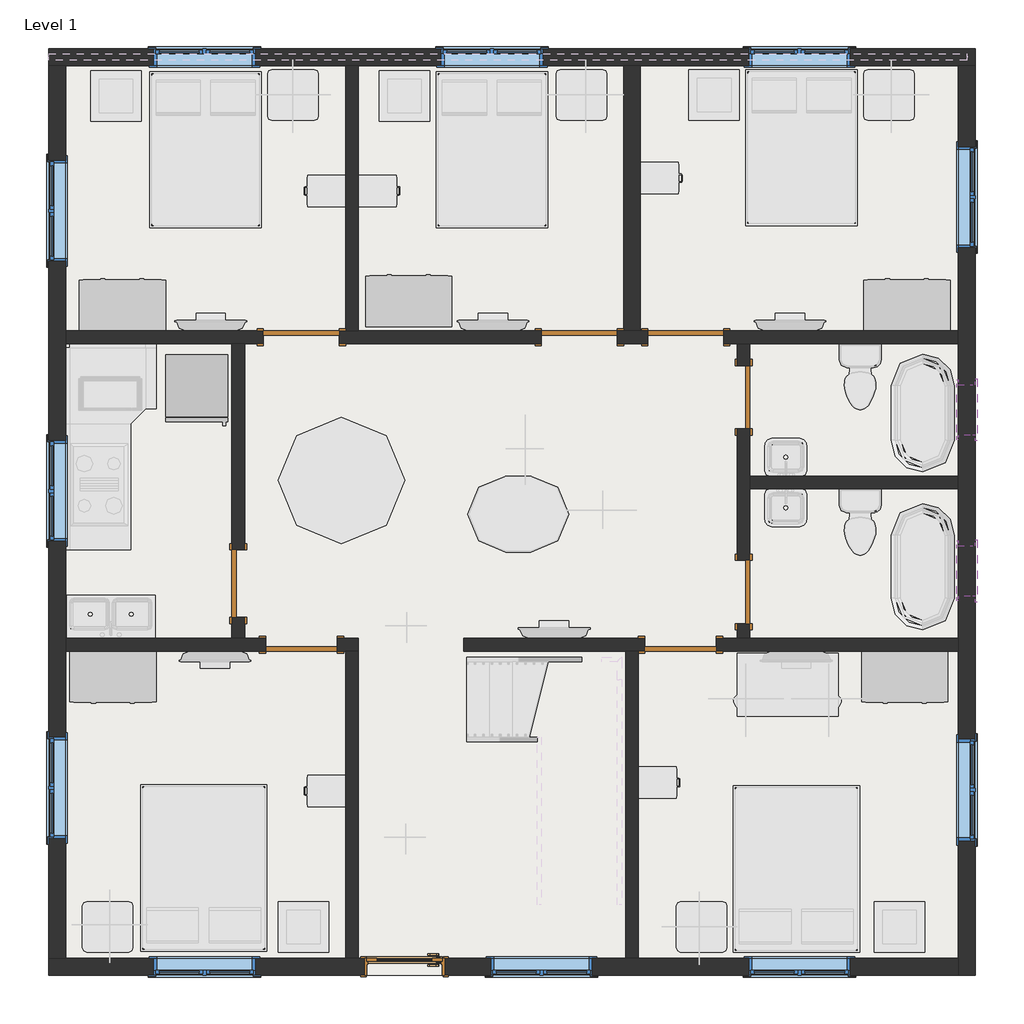
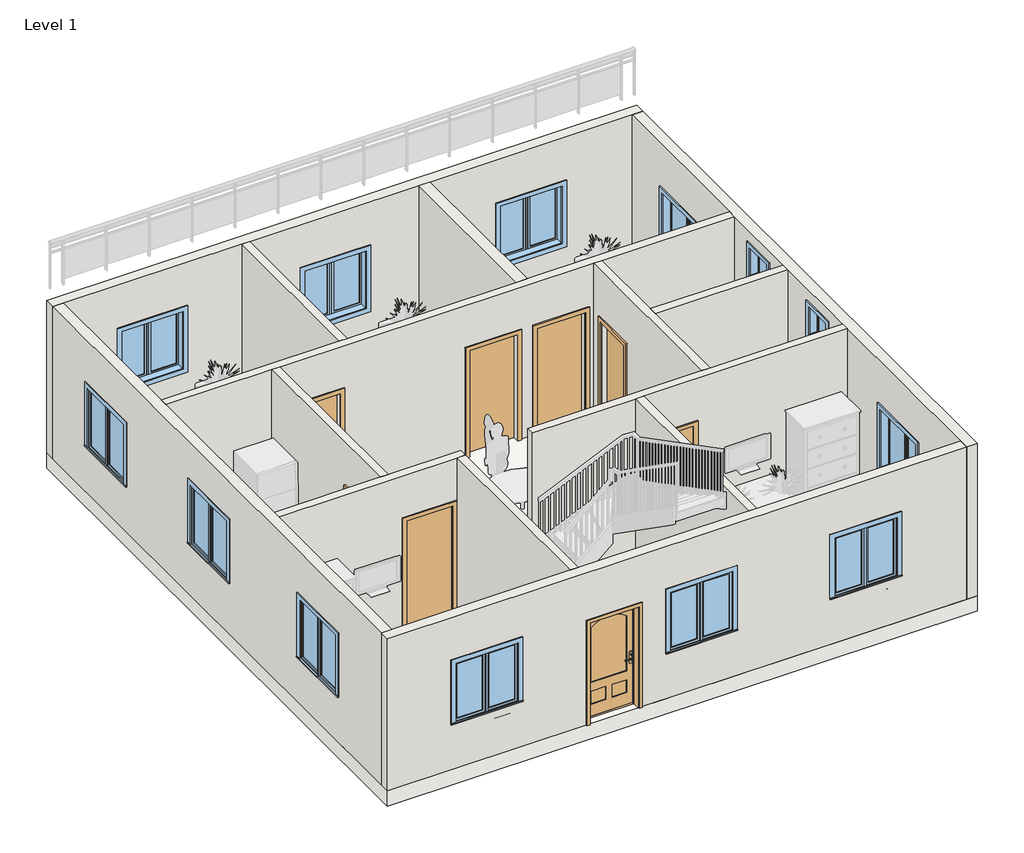
# One storey, part 1 of 3: 14 walls, 13 windows, 9 doors, 1 slab.
"""IFC4 building model written with IfcOpenShell, lengths in millimetres."""

from ifc_helpers import new_model, si_unit, frame, origin, origin_with_axes, place, context, project, spatial, polyline, outline, extrude, faceted_brep, transform, mapped, element, save
from components import door_1768e003, door_255cab33, door_059fdd7e, door_bb092f7c, door_99d96fc5, door_b6e9fca3, door_16372e1c, door_686f89d2, window_0862ab64, window_e41d21a6

model = new_model("IFC4")

# Units and contexts
model_context = context("Model", 3, world=origin())
ifc_project = project(units=[si_unit("LENGTHUNIT", "METRE", prefix="MILLI")], contexts=[model_context])

# Site, building, storey
site = spatial("IfcSite", under=ifc_project)
building = spatial("IfcBuilding", under=site)
storey = spatial("IfcBuildingStorey", under=building, Name="Level 1", Elevation=0.0)

# Doors
placement = place(None, origin())
door_shape = door_1768e003(model_context)
element("IfcDoor", 1, ObjectType="36\" x 80\"", at=placement, inside=storey, context=model_context, shape_type="MappedRepresentation", body=[
    mapped(door_shape, transform((-13267.3067057, 2339.0937882, 0.0), x_axis=(1.0, 0.0, 0.0), y_axis=(0.0, 1.0, 0.0), z_axis=(0.0, 0.0, 1.0))),
])
door_2_shape = door_255cab33(model_context)
element("IfcDoor", 2, ObjectType="Single-Flush : 30\" x 80\"", at=placement, inside=storey, context=model_context, shape_type="MappedRepresentation", body=[
    mapped(door_2_shape, transform((-9177.9067057, 9206.6187882, 0.0), x_axis=(0.0, 1.0, 0.0), y_axis=(-1.0, 0.0, 0.0), z_axis=(0.0, 0.0, 1.0))),
])
door_3_shape = door_059fdd7e(model_context)
element("IfcDoor", 3, ObjectType="Single-Flush : 30\" x 80\"", at=placement, inside=storey, context=model_context, shape_type="MappedRepresentation", body=[
    mapped(door_3_shape, transform((-9177.9067057, 6857.1187882, 0.0), x_axis=(0.0, -1.0, 0.0), y_axis=(1.0, 0.0, 0.0), z_axis=(0.0, 0.0, 1.0))),
])
door_4_shape = door_bb092f7c(model_context)
element("IfcDoor", 4, ObjectType="Single-Flush : 32\" x 84\"", at=placement, inside=storey, context=model_context, shape_type="MappedRepresentation", body=[
    mapped(door_4_shape, transform((-15273.9067057, 6958.7187882, 0.0), x_axis=(0.0, -1.0, 0.0), y_axis=(1.0, 0.0, 0.0), z_axis=(0.0, 0.0, 1.0))),
])
door_5_shape = door_99d96fc5(model_context)
element("IfcDoor", 5, ObjectType="Single-Flush : 34\" x 84\"", at=placement, inside=storey, context=model_context, shape_type="MappedRepresentation", body=[
    mapped(door_5_shape, transform((-14511.9067057, 6222.1187882, 0.0), x_axis=(1.0, 0.0, 0.0), y_axis=(0.0, 1.0, 0.0), z_axis=(0.0, 0.0, 1.0))),
])
door_6_shape = door_b6e9fca3(model_context)
element("IfcDoor", 6, ObjectType="Single-Flush : 34\" x 84\"", at=placement, inside=storey, context=model_context, shape_type="MappedRepresentation", body=[
    mapped(door_6_shape, transform((-9939.9067057, 6222.1187882, 0.0), x_axis=(-1.0, 0.0, 0.0), y_axis=(0.0, -1.0, 0.0), z_axis=(0.0, 0.0, 1.0))),
])
door_7_shape = door_16372e1c(model_context)
element("IfcDoor", 7, ObjectType="Single-Flush : 36\" x 84\"", at=placement, inside=storey, context=model_context, shape_type="MappedRepresentation", body=[
    mapped(door_7_shape, transform((-14511.9067057, 9930.5187882, 0.0), x_axis=(1.0, 0.0, 0.0), y_axis=(0.0, 1.0, 0.0), z_axis=(0.0, 0.0, 1.0))),
])
element("IfcDoor", 8, ObjectType="Single-Flush : 36\" x 84\"", at=placement, inside=storey, context=model_context, shape_type="MappedRepresentation", body=[
    mapped(door_7_shape, transform((-11159.1067057, 9930.5187882, 0.0), x_axis=(1.0, 0.0, 0.0), y_axis=(0.0, 1.0, 0.0), z_axis=(0.0, 0.0, 1.0))),
])
door_8_shape = door_686f89d2(model_context)
element("IfcDoor", 9, ObjectType="Single-Flush : 36\" x 84\"", at=placement, inside=storey, context=model_context, shape_type="MappedRepresentation", body=[
    mapped(door_8_shape, transform((-9876.4067057, 9930.5187882, 0.0), x_axis=(-1.0, 0.0, 0.0), y_axis=(0.0, -1.0, 0.0), z_axis=(0.0, 0.0, 1.0))),
])

# Slab
element("IfcSlab", 10, ObjectType="Generic - 12\"", at=placement, inside=storey, context=model_context, shape_type="SweptSolid", body=[
    extrude(outline(polyline([(-6383.9067057, 13410.3187882), (-6383.9067057, 2234.3187882), (-17559.9067057, 2234.3187882), (-17559.9067057, 13410.3187882), (-6383.9067057, 13410.3187882)])), frame((0.0, 0.0, -304.8), z_axis=(0.0, 0.0, 1.0), x_axis=(1.0, 0.0, 0.0)), (0.0, 0.0, 1.0), 304.8),
])

# Walls
element("IfcWall", 11, ObjectType="Generic - 8\"", at=placement, inside=storey, context=model_context, shape_type="Brep", body=[
    faceted_brep([(-17559.9067057, 13207.1187882, 0.0), (-17356.7067057, 13207.1187882, 0.0), (-13978.5067057, 13207.1187882, 0.0), (-13826.1067057, 13207.1187882, 0.0), (-10625.7067057, 13207.1187882, 0.0), (-10422.5067057, 13207.1187882, 0.0), (-6587.1067057, 13207.1187882, 0.0), (-6383.9067057, 13207.1187882, 0.0), (-6383.9067057, 13207.1187882, 3048.0), (-6587.1067057, 13207.1187882, 3048.0), (-10422.5067057, 13207.1187882, 3048.0), (-10625.7067057, 13207.1187882, 3048.0), (-13826.1067057, 13207.1187882, 3048.0), (-13978.5067057, 13207.1187882, 3048.0), (-17356.7067057, 13207.1187882, 3048.0), (-17559.9067057, 13207.1187882, 3048.0), (-15070.7067057, 13207.1187882, 2133.6), (-15070.7067057, 13207.1187882, 914.4), (-16289.9067057, 13207.1187882, 914.4), (-16289.9067057, 13207.1187882, 2133.6), (-11603.6067057, 13207.1187882, 2133.6), (-11603.6067057, 13207.1187882, 914.4), (-12822.8067057, 13207.1187882, 914.4), (-12822.8067057, 13207.1187882, 2133.6), (-7895.2067057, 13207.1187882, 2133.6), (-7895.2067057, 13207.1187882, 914.4), (-9114.4067057, 13207.1187882, 914.4), (-9114.4067057, 13207.1187882, 2133.6), (-17559.9067057, 13410.3187882, 0.0), (-17559.9067057, 13410.3187882, 3048.0), (-6383.9067057, 13410.3187882, 3048.0), (-6383.9067057, 13410.3187882, 0.0), (-15070.7067057, 13410.3187882, 2133.6), (-16289.9067057, 13410.3187882, 2133.6), (-16289.9067057, 13410.3187882, 914.4), (-15070.7067057, 13410.3187882, 914.4), (-11603.6067057, 13410.3187882, 2133.6), (-12822.8067057, 13410.3187882, 2133.6), (-12822.8067057, 13410.3187882, 914.4), (-11603.6067057, 13410.3187882, 914.4), (-7895.2067057, 13410.3187882, 2133.6), (-9114.4067057, 13410.3187882, 2133.6), (-9114.4067057, 13410.3187882, 914.4), (-7895.2067057, 13410.3187882, 914.4)], [[[0, 1, 2, 3, 4, 5, 6, 7, 8, 9, 10, 11, 12, 13, 14, 15], [16, 17, 18, 19], [20, 21, 22, 23], [24, 25, 26, 27]], [[28, 29, 30, 31], [32, 33, 34, 35], [36, 37, 38, 39], [40, 41, 42, 43]], [[7, 6, 5, 4, 3, 2, 1, 0, 28, 31]], [[8, 7, 31, 30]], [[0, 15, 29, 28]], [[17, 16, 32, 35]], [[18, 17, 35, 34]], [[19, 18, 34, 33]], [[16, 19, 33, 32]], [[21, 20, 36, 39]], [[22, 21, 39, 38]], [[23, 22, 38, 37]], [[20, 23, 37, 36]], [[25, 24, 40, 43]], [[26, 25, 43, 42]], [[27, 26, 42, 41]], [[24, 27, 41, 40]], [[15, 14, 13, 12, 11, 10, 9, 8, 30, 29]]]),
])
element("IfcWall", 12, ObjectType="Generic - 8\"", at=placement, inside=storey, context=model_context, shape_type="Brep", body=[
    faceted_brep([(-6587.1067057, 13207.1187882, 0.0), (-6587.1067057, 10006.7187882, 0.0), (-6587.1067057, 9854.3187882, 0.0), (-6587.1067057, 8254.1187882, 0.0), (-6587.1067057, 8101.7187882, 0.0), (-6587.1067057, 6298.3187882, 0.0), (-6587.1067057, 6145.9187882, 0.0), (-6587.1067057, 2437.5187882, 0.0), (-6587.1067057, 2234.3187882, 0.0), (-6587.1067057, 2234.3187882, 3048.0), (-6587.1067057, 2437.5187882, 3048.0), (-6587.1067057, 6145.9187882, 3048.0), (-6587.1067057, 6298.3187882, 3048.0), (-6587.1067057, 8101.7187882, 3048.0), (-6587.1067057, 8254.1187882, 3048.0), (-6587.1067057, 9854.3187882, 3048.0), (-6587.1067057, 10006.7187882, 3048.0), (-6587.1067057, 13207.1187882, 3048.0), (-6587.1067057, 3859.9187882, 2133.6), (-6587.1067057, 3859.9187882, 914.4), (-6587.1067057, 5079.1187882, 914.4), (-6587.1067057, 5079.1187882, 2133.6), (-6587.1067057, 11010.0187882, 2133.6), (-6587.1067057, 11010.0187882, 914.4), (-6587.1067057, 12229.2187882, 914.4), (-6587.1067057, 12229.2187882, 2133.6), (-6587.1067057, 8749.4187882, 2768.6), (-6587.1067057, 8749.4187882, 2159.0), (-6587.1067057, 9359.0187882, 2159.0), (-6587.1067057, 9359.0187882, 2768.6), (-6587.1067057, 6806.3187882, 2768.6), (-6587.1067057, 6806.3187882, 2159.0), (-6587.1067057, 7415.9187882, 2159.0), (-6587.1067057, 7415.9187882, 2768.6), (-6383.9067057, 13207.1187882, 0.0), (-6383.9067057, 13207.1187882, 3048.0), (-6383.9067057, 2234.3187882, 3048.0), (-6383.9067057, 2234.3187882, 0.0), (-6383.9067057, 3859.9187882, 2133.6), (-6383.9067057, 5079.1187882, 2133.6), (-6383.9067057, 5079.1187882, 914.4), (-6383.9067057, 3859.9187882, 914.4), (-6383.9067057, 11010.0187882, 2133.6), (-6383.9067057, 12229.2187882, 2133.6), (-6383.9067057, 12229.2187882, 914.4), (-6383.9067057, 11010.0187882, 914.4), (-6383.9067057, 8749.4187882, 2768.6), (-6383.9067057, 9359.0187882, 2768.6), (-6383.9067057, 9359.0187882, 2159.0), (-6383.9067057, 8749.4187882, 2159.0), (-6383.9067057, 6806.3187882, 2768.6), (-6383.9067057, 7415.9187882, 2768.6), (-6383.9067057, 7415.9187882, 2159.0), (-6383.9067057, 6806.3187882, 2159.0)], [[[0, 1, 2, 3, 4, 5, 6, 7, 8, 9, 10, 11, 12, 13, 14, 15, 16, 17], [18, 19, 20, 21], [22, 23, 24, 25], [26, 27, 28, 29], [30, 31, 32, 33]], [[34, 35, 36, 37], [38, 39, 40, 41], [42, 43, 44, 45], [46, 47, 48, 49], [50, 51, 52, 53]], [[8, 7, 6, 5, 4, 3, 2, 1, 0, 34, 37]], [[0, 17, 35, 34]], [[9, 8, 37, 36]], [[19, 18, 38, 41]], [[20, 19, 41, 40]], [[21, 20, 40, 39]], [[18, 21, 39, 38]], [[23, 22, 42, 45]], [[24, 23, 45, 44]], [[25, 24, 44, 43]], [[22, 25, 43, 42]], [[17, 16, 15, 14, 13, 12, 11, 10, 9, 36, 35]], [[27, 26, 46, 49]], [[28, 27, 49, 48]], [[29, 28, 48, 47]], [[26, 29, 47, 46]], [[31, 30, 50, 53]], [[32, 31, 53, 52]], [[33, 32, 52, 51]], [[30, 33, 51, 50]]]),
])
element("IfcWall", 13, ObjectType="Generic - 8\"", at=placement, inside=storey, context=model_context, shape_type="Brep", body=[
    faceted_brep([(-6587.1067057, 2437.5187882, 3048.0), (-6587.1067057, 2437.5187882, 0.0), (-10447.9067057, 2437.5187882, 0.0), (-10600.3067057, 2437.5187882, 0.0), (-12784.7067057, 2437.5187882, 0.0), (-12784.7067057, 2437.5187882, 2057.4), (-13749.9067057, 2437.5187882, 2057.4), (-13749.9067057, 2437.5187882, 0.0), (-13826.1067057, 2437.5187882, 0.0), (-13978.5067057, 2437.5187882, 0.0), (-17356.7067057, 2437.5187882, 0.0), (-17559.9067057, 2437.5187882, 0.0), (-17559.9067057, 2437.5187882, 3048.0), (-17356.7067057, 2437.5187882, 3048.0), (-13978.5067057, 2437.5187882, 3048.0), (-13826.1067057, 2437.5187882, 3048.0), (-10600.3067057, 2437.5187882, 3048.0), (-10447.9067057, 2437.5187882, 3048.0), (-16289.9067057, 2437.5187882, 2133.6), (-16289.9067057, 2437.5187882, 914.4), (-15070.7067057, 2437.5187882, 914.4), (-15070.7067057, 2437.5187882, 2133.6), (-12225.9067057, 2437.5187882, 2133.6), (-12225.9067057, 2437.5187882, 914.4), (-11006.7067057, 2437.5187882, 914.4), (-11006.7067057, 2437.5187882, 2133.6), (-9114.4067057, 2437.5187882, 2133.6), (-9114.4067057, 2437.5187882, 914.4), (-7895.2067057, 2437.5187882, 914.4), (-7895.2067057, 2437.5187882, 2133.6), (-6587.1067057, 2234.3187882, 0.0), (-6587.1067057, 2234.3187882, 3048.0), (-17559.9067057, 2234.3187882, 3048.0), (-17559.9067057, 2234.3187882, 0.0), (-13749.9067057, 2234.3187882, 0.0), (-13749.9067057, 2234.3187882, 2057.4), (-12784.7067057, 2234.3187882, 2057.4), (-12784.7067057, 2234.3187882, 0.0), (-16289.9067057, 2234.3187882, 2133.6), (-15070.7067057, 2234.3187882, 2133.6), (-15070.7067057, 2234.3187882, 914.4), (-16289.9067057, 2234.3187882, 914.4), (-12225.9067057, 2234.3187882, 2133.6), (-11006.7067057, 2234.3187882, 2133.6), (-11006.7067057, 2234.3187882, 914.4), (-12225.9067057, 2234.3187882, 914.4), (-9114.4067057, 2234.3187882, 2133.6), (-7895.2067057, 2234.3187882, 2133.6), (-7895.2067057, 2234.3187882, 914.4), (-9114.4067057, 2234.3187882, 914.4)], [[[0, 1, 2, 3, 4, 5, 6, 7, 8, 9, 10, 11, 12, 13, 14, 15, 16, 17], [18, 19, 20, 21], [22, 23, 24, 25], [26, 27, 28, 29]], [[30, 31, 32, 33, 34, 35, 36, 37], [38, 39, 40, 41], [42, 43, 44, 45], [46, 47, 48, 49]], [[1, 30, 37, 4, 3, 2]], [[33, 11, 10, 9, 8, 7, 34]], [[1, 0, 31, 30]], [[12, 11, 33, 32]], [[36, 5, 4, 37]], [[5, 36, 35, 6]], [[6, 35, 34, 7]], [[19, 18, 38, 41]], [[20, 19, 41, 40]], [[21, 20, 40, 39]], [[18, 21, 39, 38]], [[23, 22, 42, 45]], [[24, 23, 45, 44]], [[25, 24, 44, 43]], [[22, 25, 43, 42]], [[27, 26, 46, 49]], [[28, 27, 49, 48]], [[29, 28, 48, 47]], [[26, 29, 47, 46]], [[0, 17, 16, 15, 14, 13, 12, 32, 31]]]),
])
element("IfcWall", 14, ObjectType="Generic - 8\"", at=placement, inside=storey, context=model_context, shape_type="Brep", body=[
    faceted_brep([(-17356.7067057, 2437.5187882, 0.0), (-17356.7067057, 6145.9187882, 0.0), (-17356.7067057, 6298.3187882, 0.0), (-17356.7067057, 9854.3187882, 0.0), (-17356.7067057, 10006.7187882, 0.0), (-17356.7067057, 13207.1187882, 0.0), (-17356.7067057, 13207.1187882, 3048.0), (-17356.7067057, 10006.7187882, 3048.0), (-17356.7067057, 9854.3187882, 3048.0), (-17356.7067057, 6298.3187882, 3048.0), (-17356.7067057, 6145.9187882, 3048.0), (-17356.7067057, 2437.5187882, 3048.0), (-17356.7067057, 12064.1187882, 2133.6), (-17356.7067057, 12064.1187882, 914.4), (-17356.7067057, 10844.9187882, 914.4), (-17356.7067057, 10844.9187882, 2133.6), (-17356.7067057, 8685.9187882, 2247.9), (-17356.7067057, 8685.9187882, 1028.7), (-17356.7067057, 7466.7187882, 1028.7), (-17356.7067057, 7466.7187882, 2247.9), (-17356.7067057, 5104.5187882, 2133.6), (-17356.7067057, 5104.5187882, 914.4), (-17356.7067057, 3885.3187882, 914.4), (-17356.7067057, 3885.3187882, 2133.6), (-17559.9067057, 2437.5187882, 0.0), (-17559.9067057, 2437.5187882, 3048.0), (-17559.9067057, 13207.1187882, 3048.0), (-17559.9067057, 13207.1187882, 0.0), (-17559.9067057, 12064.1187882, 2133.6), (-17559.9067057, 10844.9187882, 2133.6), (-17559.9067057, 10844.9187882, 914.4), (-17559.9067057, 12064.1187882, 914.4), (-17559.9067057, 8685.9187882, 2247.9), (-17559.9067057, 7466.7187882, 2247.9), (-17559.9067057, 7466.7187882, 1028.7), (-17559.9067057, 8685.9187882, 1028.7), (-17559.9067057, 5104.5187882, 2133.6), (-17559.9067057, 3885.3187882, 2133.6), (-17559.9067057, 3885.3187882, 914.4), (-17559.9067057, 5104.5187882, 914.4)], [[[0, 1, 2, 3, 4, 5, 6, 7, 8, 9, 10, 11], [12, 13, 14, 15], [16, 17, 18, 19], [20, 21, 22, 23]], [[24, 25, 26, 27], [28, 29, 30, 31], [32, 33, 34, 35], [36, 37, 38, 39]], [[5, 4, 3, 2, 1, 0, 24, 27]], [[6, 5, 27, 26]], [[0, 11, 25, 24]], [[13, 12, 28, 31]], [[14, 13, 31, 30]], [[15, 14, 30, 29]], [[12, 15, 29, 28]], [[17, 16, 32, 35]], [[18, 17, 35, 34]], [[19, 18, 34, 33]], [[16, 19, 33, 32]], [[21, 20, 36, 39]], [[22, 21, 39, 38]], [[23, 22, 38, 37]], [[20, 23, 37, 36]], [[11, 10, 9, 8, 7, 6, 26, 25]]]),
])
element("IfcWall", 15, ObjectType="Generic - 8\"", at=placement, inside=storey, context=model_context, shape_type="SweptSolid", body=[
    extrude(outline(polyline([(-10625.7067057, 10006.7187882), (-10625.7067057, 13207.1187882), (-10422.5067057, 13207.1187882), (-10422.5067057, 10006.7187882), (-10625.7067057, 10006.7187882)])), origin_with_axes(), (0.0, 0.0, 1.0), 3048.0),
])
element("IfcWall", 16, ObjectType="INNER 6\"", at=placement, inside=storey, context=model_context, shape_type="Brep", body=[
    faceted_brep([(-10701.9067057, 9854.3187882, 0.0), (-10333.6067057, 9854.3187882, 0.0), (-10333.6067057, 9854.3187882, 2133.6), (-9419.2067057, 9854.3187882, 2133.6), (-9419.2067057, 9854.3187882, 0.0), (-9254.1067057, 9854.3187882, 0.0), (-9101.7067057, 9854.3187882, 0.0), (-6587.1067057, 9854.3187882, 0.0), (-6587.1067057, 9854.3187882, 3048.0), (-9101.7067057, 9854.3187882, 3048.0), (-9254.1067057, 9854.3187882, 3048.0), (-15197.7067057, 9854.3187882, 3048.0), (-15350.1067057, 9854.3187882, 3048.0), (-17356.7067057, 9854.3187882, 3048.0), (-17356.7067057, 9854.3187882, 0.0), (-15350.1067057, 9854.3187882, 0.0), (-15197.7067057, 9854.3187882, 0.0), (-14969.1067057, 9854.3187882, 0.0), (-14969.1067057, 9854.3187882, 2133.6), (-14054.7067057, 9854.3187882, 2133.6), (-14054.7067057, 9854.3187882, 0.0), (-11616.3067057, 9854.3187882, 0.0), (-11616.3067057, 9854.3187882, 2133.6), (-10701.9067057, 9854.3187882, 2133.6), (-10333.6067057, 10006.7187882, 2133.6), (-10333.6067057, 10006.7187882, 0.0), (-10422.5067057, 10006.7187882, 0.0), (-10625.7067057, 10006.7187882, 0.0), (-10701.9067057, 10006.7187882, 0.0), (-10701.9067057, 10006.7187882, 2133.6), (-11616.3067057, 10006.7187882, 2133.6), (-11616.3067057, 10006.7187882, 0.0), (-13826.1067057, 10006.7187882, 0.0), (-13978.5067057, 10006.7187882, 0.0), (-14054.7067057, 10006.7187882, 0.0), (-14054.7067057, 10006.7187882, 2133.6), (-14969.1067057, 10006.7187882, 2133.6), (-14969.1067057, 10006.7187882, 0.0), (-17356.7067057, 10006.7187882, 0.0), (-17356.7067057, 10006.7187882, 3048.0), (-13978.5067057, 10006.7187882, 3048.0), (-13826.1067057, 10006.7187882, 3048.0), (-10625.7067057, 10006.7187882, 3048.0), (-10422.5067057, 10006.7187882, 3048.0), (-6587.1067057, 10006.7187882, 3048.0), (-6587.1067057, 10006.7187882, 0.0), (-9419.2067057, 10006.7187882, 0.0), (-9419.2067057, 10006.7187882, 2133.6)], [[[0, 1, 2, 3, 4, 5, 6, 7, 8, 9, 10, 11, 12, 13, 14, 15, 16, 17, 18, 19, 20, 21, 22, 23]], [[24, 25, 26, 27, 28, 29, 30, 31, 32, 33, 34, 35, 36, 37, 38, 39, 40, 41, 42, 43, 44, 45, 46, 47]], [[17, 16, 15, 14, 38, 37]], [[21, 20, 34, 33, 32, 31]], [[46, 45, 7, 6, 5, 4]], [[28, 27, 26, 25, 1, 0]], [[8, 7, 45, 44]], [[14, 13, 39, 38]], [[35, 34, 20, 19]], [[36, 35, 19, 18]], [[37, 36, 18, 17]], [[29, 28, 0, 23]], [[30, 29, 23, 22]], [[31, 30, 22, 21]], [[2, 1, 25, 24]], [[3, 2, 24, 47]], [[4, 3, 47, 46]], [[13, 12, 11, 10, 9, 8, 44, 43, 42, 41, 40, 39]]]),
])
element("IfcWall", 17, ObjectType="INNER 6\"", at=placement, inside=storey, context=model_context, shape_type="SweptSolid", body=[
    extrude(outline(polyline([(6552.3187882, 2133.6), (6552.3187882, 0.0), (6298.3187882, 0.0), (6298.3187882, 3048.0), (9854.3187882, 3048.0), (9854.3187882, 0.0), (7365.1187882, 0.0), (7365.1187882, 2133.6), (6552.3187882, 2133.6)])), frame((-15350.1067057, 0.0, 0.0), z_axis=(1.0, 0.0, 0.0), x_axis=(0.0, 1.0, 0.0)), (0.0, 0.0, 1.0), 152.4),
])
element("IfcWall", 18, ObjectType="INNER 6\"", at=placement, inside=storey, context=model_context, shape_type="Brep", body=[
    faceted_brep([(-9254.1067057, 6476.1187882, 2032.0), (-9254.1067057, 6476.1187882, 0.0), (-9254.1067057, 6298.3187882, 0.0), (-9254.1067057, 6298.3187882, 3048.0), (-9254.1067057, 9854.3187882, 3048.0), (-9254.1067057, 9854.3187882, 0.0), (-9254.1067057, 9587.6187882, 0.0), (-9254.1067057, 9587.6187882, 2032.0), (-9254.1067057, 8825.6187882, 2032.0), (-9254.1067057, 8825.6187882, 0.0), (-9254.1067057, 7238.1187882, 0.0), (-9254.1067057, 7238.1187882, 2032.0), (-9101.7067057, 6298.3187882, 0.0), (-9101.7067057, 6476.1187882, 0.0), (-9101.7067057, 6476.1187882, 2032.0), (-9101.7067057, 7238.1187882, 2032.0), (-9101.7067057, 7238.1187882, 0.0), (-9101.7067057, 8101.7187882, 0.0), (-9101.7067057, 8254.1187882, 0.0), (-9101.7067057, 8825.6187882, 0.0), (-9101.7067057, 8825.6187882, 2032.0), (-9101.7067057, 9587.6187882, 2032.0), (-9101.7067057, 9587.6187882, 0.0), (-9101.7067057, 9854.3187882, 0.0), (-9101.7067057, 9854.3187882, 3048.0), (-9101.7067057, 8254.1187882, 3048.0), (-9101.7067057, 8101.7187882, 3048.0), (-9101.7067057, 6298.3187882, 3048.0)], [[[0, 1, 2, 3, 4, 5, 6, 7, 8, 9, 10, 11]], [[12, 13, 14, 15, 16, 17, 18, 19, 20, 21, 22, 23, 24, 25, 26, 27]], [[23, 22, 6, 5]], [[10, 9, 19, 18, 17, 16]], [[2, 1, 13, 12]], [[5, 4, 24, 23]], [[3, 2, 12, 27]], [[7, 6, 22, 21]], [[8, 7, 21, 20]], [[9, 8, 20, 19]], [[14, 13, 1, 0]], [[15, 14, 0, 11]], [[16, 15, 11, 10]], [[4, 3, 27, 26, 25, 24]]]),
])
element("IfcWall", 19, ObjectType="INNER 6\"", at=placement, inside=storey, context=model_context, shape_type="Brep", body=[
    faceted_brep([(-14080.1067057, 6145.9187882, 2133.6), (-14080.1067057, 6145.9187882, 0.0), (-13978.5067057, 6145.9187882, 0.0), (-13826.1067057, 6145.9187882, 0.0), (-13826.1067057, 6145.9187882, 3048.0), (-13978.5067057, 6145.9187882, 3048.0), (-17356.7067057, 6145.9187882, 3048.0), (-17356.7067057, 6145.9187882, 0.0), (-14943.7067057, 6145.9187882, 0.0), (-14943.7067057, 6145.9187882, 2133.6), (-13826.1067057, 6298.3187882, 0.0), (-14080.1067057, 6298.3187882, 0.0), (-14080.1067057, 6298.3187882, 2133.6), (-14943.7067057, 6298.3187882, 2133.6), (-14943.7067057, 6298.3187882, 0.0), (-15197.7067057, 6298.3187882, 0.0), (-15350.1067057, 6298.3187882, 0.0), (-17356.7067057, 6298.3187882, 0.0), (-17356.7067057, 6298.3187882, 3048.0), (-15350.1067057, 6298.3187882, 3048.0), (-15197.7067057, 6298.3187882, 3048.0), (-13826.1067057, 6298.3187882, 3048.0)], [[[0, 1, 2, 3, 4, 5, 6, 7, 8, 9]], [[10, 11, 12, 13, 14, 15, 16, 17, 18, 19, 20, 21]], [[8, 7, 17, 16, 15, 14]], [[3, 2, 1, 11, 10]], [[7, 6, 18, 17]], [[12, 11, 1, 0]], [[13, 12, 0, 9]], [[14, 13, 9, 8]], [[4, 3, 10, 21]], [[6, 5, 4, 21, 20, 19, 18]]]),
])
element("IfcWall", 20, ObjectType="INNER 6\"", at=placement, inside=storey, context=model_context, shape_type="SweptSolid", body=[
    extrude(outline(polyline([(-13978.5067057, 10006.7187882), (-13978.5067057, 13207.1187882), (-13826.1067057, 13207.1187882), (-13826.1067057, 10006.7187882), (-13978.5067057, 10006.7187882)])), origin_with_axes(), (0.0, 0.0, 1.0), 3048.0),
])
element("IfcWall", 21, ObjectType="INNER 6\"", at=placement, inside=storey, context=model_context, shape_type="SweptSolid", body=[
    extrude(outline(polyline([(-6587.1067057, 8101.7187882), (-9101.7067057, 8101.7187882), (-9101.7067057, 8254.1187882), (-6587.1067057, 8254.1187882), (-6587.1067057, 8101.7187882)])), origin_with_axes(), (0.0, 0.0, 1.0), 3048.0),
])
element("IfcWall", 22, ObjectType="INNER 6\"", at=placement, inside=storey, context=model_context, shape_type="SweptSolid", body=[
    extrude(outline(polyline([(-13978.5067057, 2437.5187882), (-13978.5067057, 6145.9187882), (-13826.1067057, 6145.9187882), (-13826.1067057, 2437.5187882), (-13978.5067057, 2437.5187882)])), origin_with_axes(), (0.0, 0.0, 1.0), 3048.0),
])
element("IfcWall", 23, ObjectType="INNER 6\"", at=placement, inside=storey, context=model_context, shape_type="SweptSolid", body=[
    extrude(outline(polyline([(-10600.3067057, 2437.5187882), (-10600.3067057, 6145.9187882), (-10447.9067057, 6145.9187882), (-10447.9067057, 2437.5187882), (-10600.3067057, 2437.5187882)])), origin_with_axes(), (0.0, 0.0, 1.0), 3048.0),
])
element("IfcWall", 24, ObjectType="INNER 6\"", at=placement, inside=storey, context=model_context, shape_type="Brep", body=[
    faceted_brep([(-12556.1067057, 6145.9187882, 0.0), (-10600.3067057, 6145.9187882, 0.0), (-10447.9067057, 6145.9187882, 0.0), (-10371.7067057, 6145.9187882, 0.0), (-10371.7067057, 6145.9187882, 2133.6), (-9508.1067057, 6145.9187882, 2133.6), (-9508.1067057, 6145.9187882, 0.0), (-6587.1067057, 6145.9187882, 0.0), (-6587.1067057, 6145.9187882, 3048.0), (-10447.9067057, 6145.9187882, 3048.0), (-10600.3067057, 6145.9187882, 3048.0), (-12556.1067057, 6145.9187882, 3048.0), (-10371.7067057, 6298.3187882, 2133.6), (-10371.7067057, 6298.3187882, 0.0), (-12556.1067057, 6298.3187882, 0.0), (-12556.1067057, 6298.3187882, 3048.0), (-9254.1067057, 6298.3187882, 3048.0), (-9101.7067057, 6298.3187882, 3048.0), (-6587.1067057, 6298.3187882, 3048.0), (-6587.1067057, 6298.3187882, 0.0), (-9101.7067057, 6298.3187882, 0.0), (-9254.1067057, 6298.3187882, 0.0), (-9508.1067057, 6298.3187882, 0.0), (-9508.1067057, 6298.3187882, 2133.6)], [[[0, 1, 2, 3, 4, 5, 6, 7, 8, 9, 10, 11]], [[12, 13, 14, 15, 16, 17, 18, 19, 20, 21, 22, 23]], [[14, 13, 3, 2, 1, 0]], [[22, 21, 20, 19, 7, 6]], [[0, 11, 15, 14]], [[8, 7, 19, 18]], [[6, 5, 23, 22]], [[5, 4, 12, 23]], [[4, 3, 13, 12]], [[11, 10, 9, 8, 18, 17, 16, 15]]]),
])

# Windows
window_shape = window_0862ab64(model_context)
element("IfcWindow", 25, ObjectType="Casement Dbl with Trim : 48\" x 48\"", at=placement, inside=storey, context=model_context, shape_type="MappedRepresentation", body=[
    mapped(window_shape, transform((-15680.3067057, 13289.6687882, 0.0), x_axis=(1.0, 0.0, 0.0), y_axis=(0.0, 1.0, 0.0), z_axis=(0.0, 0.0, 1.0))),
])
element("IfcWindow", 26, ObjectType="Casement Dbl with Trim : 48\" x 48\"", at=placement, inside=storey, context=model_context, shape_type="MappedRepresentation", body=[
    mapped(window_shape, transform((-17439.2567057, 11454.5187882, 0.0), x_axis=(0.0, 1.0, 0.0), y_axis=(-1.0, 0.0, 0.0), z_axis=(0.0, 0.0, 1.0))),
])
element("IfcWindow", 27, ObjectType="Casement Dbl with Trim : 48\" x 48\"", at=placement, inside=storey, context=model_context, shape_type="MappedRepresentation", body=[
    mapped(window_shape, transform((-17439.2567057, 8076.3187882, 114.3), x_axis=(0.0, 1.0, 0.0), y_axis=(-1.0, 0.0, 0.0), z_axis=(0.0, 0.0, 1.0))),
])
element("IfcWindow", 28, ObjectType="Casement Dbl with Trim : 48\" x 48\"", at=placement, inside=storey, context=model_context, shape_type="MappedRepresentation", body=[
    mapped(window_shape, transform((-17439.2567057, 4494.9187882, 0.0), x_axis=(0.0, 1.0, 0.0), y_axis=(-1.0, 0.0, 0.0), z_axis=(0.0, 0.0, 1.0))),
])
element("IfcWindow", 29, ObjectType="Casement Dbl with Trim : 48\" x 48\"", at=placement, inside=storey, context=model_context, shape_type="MappedRepresentation", body=[
    mapped(window_shape, transform((-15680.3067057, 2354.9687882, 0.0), x_axis=(-1.0, 0.0, 0.0), y_axis=(0.0, -1.0, 0.0), z_axis=(0.0, 0.0, 1.0))),
])
element("IfcWindow", 30, ObjectType="Casement Dbl with Trim : 48\" x 48\"", at=placement, inside=storey, context=model_context, shape_type="MappedRepresentation", body=[
    mapped(window_shape, transform((-11616.3067057, 2354.9687882, 0.0), x_axis=(-1.0, 0.0, 0.0), y_axis=(0.0, -1.0, 0.0), z_axis=(0.0, 0.0, 1.0))),
])
element("IfcWindow", 31, ObjectType="Casement Dbl with Trim : 48\" x 48\"", at=placement, inside=storey, context=model_context, shape_type="MappedRepresentation", body=[
    mapped(window_shape, transform((-8504.8067057, 2354.9687882, 0.0), x_axis=(-1.0, 0.0, 0.0), y_axis=(0.0, -1.0, 0.0), z_axis=(0.0, 0.0, 1.0))),
])
element("IfcWindow", 32, ObjectType="Casement Dbl with Trim : 48\" x 48\"", at=placement, inside=storey, context=model_context, shape_type="MappedRepresentation", body=[
    mapped(window_shape, transform((-6504.5567057, 4469.5187882, 0.0), x_axis=(0.0, -1.0, 0.0), y_axis=(1.0, 0.0, 0.0), z_axis=(0.0, 0.0, 1.0))),
])
element("IfcWindow", 33, ObjectType="Casement Dbl with Trim : 48\" x 48\"", at=placement, inside=storey, context=model_context, shape_type="MappedRepresentation", body=[
    mapped(window_shape, transform((-12213.2067057, 13289.6687882, 0.0), x_axis=(1.0, 0.0, 0.0), y_axis=(0.0, 1.0, 0.0), z_axis=(0.0, 0.0, 1.0))),
])
element("IfcWindow", 34, ObjectType="Casement Dbl with Trim : 48\" x 48\"", at=placement, inside=storey, context=model_context, shape_type="MappedRepresentation", body=[
    mapped(window_shape, transform((-8504.8067057, 13289.6687882, 0.0), x_axis=(1.0, 0.0, 0.0), y_axis=(0.0, 1.0, 0.0), z_axis=(0.0, 0.0, 1.0))),
])
element("IfcWindow", 35, ObjectType="Casement Dbl with Trim : 48\" x 48\"", at=placement, inside=storey, context=model_context, shape_type="MappedRepresentation", body=[
    mapped(window_shape, transform((-6504.5567057, 11619.6187882, 0.0), x_axis=(0.0, -1.0, 0.0), y_axis=(1.0, 0.0, 0.0), z_axis=(0.0, 0.0, 1.0))),
])
window_2_shape = window_e41d21a6(model_context)
element("IfcWindow", 36, ObjectType="Transom with Trim : 24\" x 24\"", at=placement, inside=storey, context=model_context, shape_type="MappedRepresentation", body=[
    mapped(window_2_shape, transform((-6485.5067057, 9016.1187882, 0.0), x_axis=(0.0, -1.0, 0.0), y_axis=(1.0, 0.0, 0.0), z_axis=(0.0, 0.0, 1.0))),
])
element("IfcWindow", 37, ObjectType="Transom with Trim : 24\" x 24\"", at=placement, inside=storey, context=model_context, shape_type="MappedRepresentation", body=[
    mapped(window_2_shape, transform((-6485.5067057, 7073.0187882, 0.0), x_axis=(0.0, -1.0, 0.0), y_axis=(1.0, 0.0, 0.0), z_axis=(0.0, 0.0, 1.0))),
])

save(model, "model.ifc")

# Revit data of these elements
# Type "36\" x 80\""
#   Type Mark = "8"
#   Assembly Code = "B2030100"
#   Analytic Construction = "French door, wood frame with single glass"
#   Threshold Offset [instance default] = 0' - 0 1/2"
#   Thickness = 0' - 1 3/8"
#   Thermal Resistance (R) = 1.0696 (h·ft²·°F)/BTU
#   Swing Angle [instance default] = 90.00°
#   Stiles = 0' - 4 3/4"
#   Rough Width = 3' - 2"
#   Rough Height = 6' - 9"
#   Radius = 1' - 8.05625"
#   Lock Rail = 0' - 7 1/8"
#   Height = 6' - 8"
#   Width = 3' - 0"
#   Heat Transfer Coefficient (U) = 0.9350 BTU/(h·ft²·°F)
#   Door Offset [instance default] = 0' - 0"
#   Bottom Rail = 0' - 9 1/2"
#   Threshold [instance default] = yes
#   Function = 1
#   Exterior Trim [instance default] = yes
#   Trim Material = Cherry
#   Threshold Material = Cherry
#   Panel Material = Cherry
#   Glazing = Glass
#   Frame Material = Cherry
#   Door Handle Material = Aluminum
#   Visual Light Transmittance = 0
#   Solar Heat Gain Coefficient = 0
#   Wall Closure = (empty or 0)
#   Construction Type = (empty or 0)
# Type "Single-Flush : 30\" x 80\""
#   Type Mark = "5"
#   Construction Type Id = "MDOOR"
#   Assembly Code = "C1020"
#   Analytic Construction = "Metal"
#   Thickness = 0' - 2"
#   Heat Transfer Coefficient (U) = 0.651978 BTU/(h·ft²·°F)
#   Height = 6' - 8"
#   Trim Projection Ext = 0' - 1"
#   Trim Projection Int = 0' - 1"
#   Trim Width = 0' - 3"
#   Width = 2' - 6"
#   Define Thermal Properties by = 1
#   Door Material = Door - Panel
#   Frame Material = Door - Frame
#   Visual Light Transmittance = 0
#   Solar Heat Gain Coefficient = 0
#   Function = (empty or 0)
#   Wall Closure = (empty or 0)
# Type "Single-Flush : 32\" x 84\""
#   Type Mark = "3"
#   Construction Type Id = "MDOOR"
#   Assembly Code = "C1020"
#   Analytic Construction = "Metal"
#   Thickness = 0' - 2"
#   Heat Transfer Coefficient (U) = 0.651978 BTU/(h·ft²·°F)
#   Height = 7' - 0"
#   Trim Projection Ext = 0' - 1"
#   Trim Projection Int = 0' - 1"
#   Trim Width = 0' - 3"
#   Width = 2' - 8"
#   Define Thermal Properties by = 1
#   Door Material = Door - Panel
#   Frame Material = Door - Frame
#   Visual Light Transmittance = 0
#   Solar Heat Gain Coefficient = 0
#   Function = (empty or 0)
#   Wall Closure = (empty or 0)
# Type "Single-Flush : 34\" x 84\""
#   Type Mark = "2"
#   Construction Type Id = "MDOOR"
#   Assembly Code = "C1020"
#   Analytic Construction = "Metal"
#   Thickness = 0' - 2"
#   Heat Transfer Coefficient (U) = 0.651978 BTU/(h·ft²·°F)
#   Height = 7' - 0"
#   Trim Projection Ext = 0' - 1"
#   Trim Projection Int = 0' - 1"
#   Trim Width = 0' - 3"
#   Width = 2' - 10"
#   Define Thermal Properties by = 1
#   Door Material = Door - Panel
#   Frame Material = Door - Frame
#   Visual Light Transmittance = 0
#   Solar Heat Gain Coefficient = 0
#   Function = (empty or 0)
#   Wall Closure = (empty or 0)
# Type "Single-Flush : 36\" x 84\""
#   Type Mark = "1"
#   Construction Type Id = "MDOOR"
#   Assembly Code = "C1020"
#   Analytic Construction = "Metal"
#   Thickness = 0' - 2"
#   Heat Transfer Coefficient (U) = 0.651978 BTU/(h·ft²·°F)
#   Height = 7' - 0"
#   Trim Projection Ext = 0' - 1"
#   Trim Projection Int = 0' - 1"
#   Trim Width = 0' - 3"
#   Width = 3' - 0"
#   Define Thermal Properties by = 1
#   Door Material = Door - Panel
#   Frame Material = Door - Frame
#   Visual Light Transmittance = 0
#   Solar Heat Gain Coefficient = 0
#   Function = (empty or 0)
#   Wall Closure = (empty or 0)
# Type "Generic - 12\""
#   Assembly Code = "B1010"
#   Function = 0
#   Layers, outside or top first: 1' - 0" no material (function 1)
# Type "Generic - 8\""
#   Assembly Code = "B2010"
#   Layers, outside or top first: 0' - 8" "Brick, Common" (function 1)
# Type "INNER 6\""
#   Assembly Code = "B2010"
#   Layers, outside or top first: 0' - 6" "Brick, Common" (function 1)
# Type "Casement Dbl with Trim : 48\" x 48\""
#   Type Mark = "10"
#   Construction Type Id = "GSP4R"
#   Assembly Code = "B2020100"
#   Analytic Construction = "1/8 in Pilkington single glazing"
#   Visual Light Transmittance = 0.9
#   Solar Heat Gain Coefficient = 0.78
#   Heat Transfer Coefficient (U) = 0.6496 BTU/(h·ft²·°F)
#   Height = 4' - 0"
#   Default Sill Height = 3' - 0"
#   Trim Projection - Ext. = 0' - 0 1/2"
#   Trim Projection - Int. = 0' - 0 3/4"
#   Trim Width - Exterior = 0' - 3 1/2"
#   Trim Width - Interior = 0' - 3 1/2"
#   Width = 4' - 0"
#   Window Inset = 0' - 0 3/4"
#   Define Thermal Properties by = 1
#   Glass Pane Material = Glass
#   Sash Material = Sash
#   Trim Exterior Material = Trim
#   Trim Interior Material = Trim
#   Wall Closure = (empty or 0)
# Type "Transom with Trim : 24\" x 24\""
#   Type Mark = "13"
#   Construction Type Id = "GSP4R"
#   Assembly Code = "B2020100"
#   Analytic Construction = "1/8 in Pilkington single glazing"
#   Visual Light Transmittance = 0.9
#   Solar Heat Gain Coefficient = 0.78
#   Heat Transfer Coefficient (U) = 0.6496 BTU/(h·ft²·°F)
#   Height = 2' - 0"
#   Default Sill Height = 7' - 1"
#   Trim Projection - Ext. = 0' - 0 1/2"
#   Trim Projection - Int. = 0' - 0 3/4"
#   Trim Width - Exterior = 0' - 3 1/2"
#   Trim Width - Interior = 0' - 3 1/2"
#   Width = 2' - 0"
#   Window Inset = 0' - 0 3/4"
#   Define Thermal Properties by = 1
#   Glass Pane Material = Glass
#   Sash Material = Sash
#   Trim Exterior Material = Trim
#   Trim Interior Material = Trim
#   Wall Closure = (empty or 0)
# Element 1 (IfcDoor, "36\" x 80\"")
#   Threshold Offset = 0' - 0 1/2"
#   Swing Angle = 90.00°
#   Door Offset = 0' - 0"
#   Threshold = yes
#   Exterior Trim = yes
#   Phase Created = New Construction
#   Materials on its faces: "Cherry", "Aluminum", "Glass"
# Elements 2, 3 (IfcDoor, "Single-Flush : 30\" x 80\"")
#   Phase Created = New Construction
#   Materials on its faces: "Door - Frame", "Door - Panel"
# Element 4 (IfcDoor, "Single-Flush : 32\" x 84\"")
#   Phase Created = New Construction
#   Materials on its faces: "Door - Frame", "Door - Panel"
# Elements 5, 6 (IfcDoor, "Single-Flush : 34\" x 84\"")
#   Phase Created = New Construction
#   Materials on its faces: "Door - Frame", "Door - Panel"
# Elements 7, 8, 9 (IfcDoor, "Single-Flush : 36\" x 84\"")
#   Phase Created = New Construction
#   Materials on its faces: "Door - Frame", "Door - Panel"
# Element 10 (IfcSlab, "Generic - 12\"")
#   Height Offset From Level = 0' - 0"
#   Phase Created = New Construction
#   Materials on its faces: "Default Floor"
# Elements 11, 12, 13, 14, 15 (IfcWall, "Generic - 8\"")
#   Top Offset = 0' - 0"
#   Base Offset = 0' - 0"
#   Unconnected Height = 10' - 0"
#   wall height = 10' - 0"
#   Phase Created = New Construction
#   Base Constraint = Level 1
#   Materials on its faces: "Brick, Common"
# Elements 16, 17, 18, 19, 20, 21, 22, 23, 24 (IfcWall, "INNER 6\"")
#   Top Offset = 0' - 0"
#   Base Offset = 0' - 0"
#   Unconnected Height = 10' - 0"
#   wall height = 10' - 0"
#   Phase Created = New Construction
#   Base Constraint = Level 1
#   Materials on its faces: "Brick, Common"
# Element 25 (IfcWindow, "Casement Dbl with Trim : 48\" x 48\"")
#   Mark = "1"
#   Phase Created = New Construction
#   Materials on its faces: "Sash", "Trim", "Glass"
# Element 26 (IfcWindow, "Casement Dbl with Trim : 48\" x 48\"")
#   Mark = "2"
#   Phase Created = New Construction
#   Materials on its faces: "Sash", "Trim", "Glass"
# Element 27 (IfcWindow, "Casement Dbl with Trim : 48\" x 48\"")
#   Mark = "3"
#   Phase Created = New Construction
#   Materials on its faces: "Sash", "Trim", "Glass"
# Element 28 (IfcWindow, "Casement Dbl with Trim : 48\" x 48\"")
#   Mark = "4"
#   Phase Created = New Construction
#   Materials on its faces: "Sash", "Trim", "Glass"
# Element 29 (IfcWindow, "Casement Dbl with Trim : 48\" x 48\"")
#   Mark = "5"
#   Phase Created = New Construction
#   Materials on its faces: "Sash", "Trim", "Glass"
# Element 30 (IfcWindow, "Casement Dbl with Trim : 48\" x 48\"")
#   Mark = "6"
#   Phase Created = New Construction
#   Materials on its faces: "Sash", "Trim", "Glass"
# Element 31 (IfcWindow, "Casement Dbl with Trim : 48\" x 48\"")
#   Mark = "7"
#   Phase Created = New Construction
#   Materials on its faces: "Sash", "Trim", "Glass"
# Element 32 (IfcWindow, "Casement Dbl with Trim : 48\" x 48\"")
#   Mark = "8"
#   Phase Created = New Construction
#   Materials on its faces: "Sash", "Trim", "Glass"
# Element 33 (IfcWindow, "Casement Dbl with Trim : 48\" x 48\"")
#   Mark = "10"
#   Phase Created = New Construction
#   Materials on its faces: "Sash", "Trim", "Glass"
# Element 34 (IfcWindow, "Casement Dbl with Trim : 48\" x 48\"")
#   Mark = "11"
#   Phase Created = New Construction
#   Materials on its faces: "Sash", "Trim", "Glass"
# Element 35 (IfcWindow, "Casement Dbl with Trim : 48\" x 48\"")
#   Mark = "12"
#   Phase Created = New Construction
#   Materials on its faces: "Sash", "Trim", "Glass"
# Element 36 (IfcWindow, "Transom with Trim : 24\" x 24\"")
#   Mark = "13"
#   Phase Created = New Construction
#   Materials on its faces: "Sash", "Trim", "Glass"
# Element 37 (IfcWindow, "Transom with Trim : 24\" x 24\"")
#   Mark = "14"
#   Phase Created = New Construction
#   Materials on its faces: "Sash", "Trim", "Glass"
# Materials
#   "Cherry": class "Wood", colour RGB 226 177 128, transparency 0, Description = "Prunus Serotina", Cost = 0
#   "Glass": class "Glass", colour RGB 0 128 192, transparency 0.75, Description = "Soda Lime Glass", Cost = 0
#   "Aluminum": class "Metal", colour RGB 247 247 247, transparency 0, Description = "Aluminum 6061", Cost = 0
#   "Door - Panel": class "Wood", colour RGB 210 159 95, transparency 0
#   "Door - Frame": colour RGB 118 70 51, transparency 0
#   "Brick, Common": class "Masonry", colour RGB 170 98 104, transparency 0, Description = "Common brick", Cost = 0
#   "Sash": class "Wood", colour RGB 224 178 126, transparency 0
#   "Trim": class "Wood", colour RGB 224 178 126, transparency 0
#   "Default Floor": colour RGB 128 128 128, transparency 0
# Room at (-15495.836, 11681.258) mm, phase "New Construction", upper level "Level 1", upper offset 10' - 0", lower offset 0' - 0"
#   Number = "1"
#   Name = "BEDROOM-3"
# Room at (-12125.104, 11528.858) mm, phase "New Construction", upper level "Level 1", upper offset 10' - 0", lower offset 0' - 0"
#   Number = "2"
#   Name = "BEDROOM-4"
# Room at (-8421.025, 11528.858) mm, phase "New Construction", upper level "Level 1", upper offset 10' - 0", lower offset 0' - 0"
#   Number = "3"
#   Name = "BEDROOM-5"
# Room at (-16305.725, 7879.925) mm, phase "New Construction", upper level "Level 1", upper offset 10' - 0", lower offset 0' - 0"
#   Number = "4"
#   Name = "KITCHEN"
# Room at (-15748.548, 3954.436) mm, phase "New Construction", upper level "Level 1", upper offset 10' - 0", lower offset 0' - 0"
#   Number = "5"
#   Name = "BEDROOM-2"
# Room at (-7809.738, 7202.168) mm, phase "New Construction", upper level "Level 1", upper offset 10' - 0", lower offset 0' - 0"
#   Number = "6"
#   Name = "TOILET-BATH"
# Room at (-7911.066, 8809.863) mm, phase "New Construction", upper level "Level 1", upper offset 10' - 0", lower offset 0' - 0"
#   Number = "7"
#   Name = "TOILET/BATH"
# Room at (-8783.465, 3954.436) mm, phase "New Construction", upper level "Level 1", upper offset 10' - 0", lower offset 0' - 0"
#   Number = "8"
#   Name = "BEDROOM-1"
# Room at (-12487.544, 7879.925) mm, phase "New Construction", upper level "Level 1", upper offset 10' - 0", lower offset 0' - 0"
#   Number = "9"
#   Name = "DINING/LIVING ROOM"
